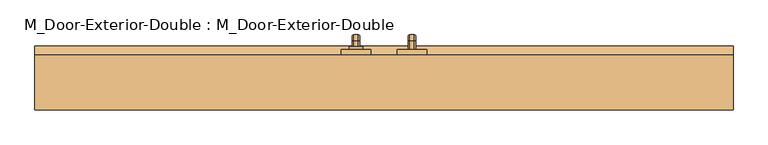
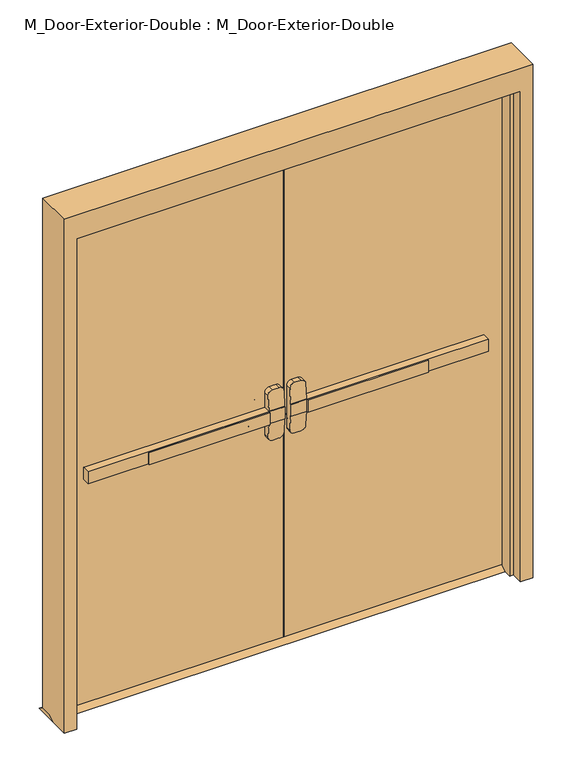
"""IFC4 building model written with IfcOpenShell, lengths in millimetres: door geometry, M_Door-Exterior-Double : M_Door-Exterior-Double."""

from ifc_helpers import new_model, si_unit, point, frame, frame_2d, origin, place, context, project, spatial, polyline, circle_curve, ellipse_curve, trimmed, segment, composite_curve, outline, extrude, faceted_brep, source, transform, mapped, element, save
from ifc_brep_helpers import plane_surface, cylinder_surface, revolved_surface, advanced_brep


def m_door_exterior_double_m_door_exterior_double_5cdccef0(model_context):
    return source(origin(), model_context, "Body", "SolidModel", [
        extrude(outline(polyline([(-566.1333333, -1.75), (-566.1333333, 4.6), (-76.2, 4.6), (-76.2, -1.75), (-566.1333333, -1.75)])), frame((0.0, 0.0, 974.6), z_axis=(0.0, 0.0, 1.0), x_axis=(1.0, 0.0, 0.0)), (0.0, 0.0, 1.0), 50.8),
        advanced_brep(
        [(-12.7, 4.6, 1025.4), (-76.2, 4.6, 1025.4), (-811.1, 4.6, 1025.4), (-811.1, 4.6, 974.6), (-76.2, 4.6, 974.6), (-12.7, 4.6, 974.6), (-811.1, 36.35, 1025.4), (-76.2, 36.35, 1025.4), (-76.2, 36.35, 1088.9), (-57.15, 36.35, 1107.95), (-31.75, 36.35, 1107.95), (-12.7, 36.35, 1088.9), (-12.7, 36.35, 911.1), (-31.75, 36.35, 892.05), (-57.15, 36.35, 892.05), (-76.2, 36.35, 911.1), (-76.2, 36.35, 974.6), (-811.1, 36.35, 974.6), (-12.7, 7.7752467, 1025.4), (-76.2, 7.7752467, 1025.4), (-12.7, 7.7752467, 974.6), (-12.7, 12.7854269, 911.1), (-12.7, 12.7854269, 1088.9), (-76.2, 7.7752467, 974.6), (-76.2, 12.7854269, 1088.9), (-76.2, 12.7854269, 911.1), (-57.15, 14.288481, 1107.95), (-31.75, 14.288481, 1107.95), (-31.75, 14.288481, 892.05), (-57.15, 14.288481, 892.05)],
        [
            (0, 1),
            (1, 2),
            (2, 3),
            (3, 4),
            (4, 5),
            (5, 0),
            (6, 7),
            (7, 8),
            (8, 9, circle_curve(frame((-57.15, 36.35, 1088.9), z_axis=(0.0, 1.0, 0.0), x_axis=(-1.0, 0.0, 0.0)), 19.05)),
            (9, 10),
            (10, 11, circle_curve(frame((-31.75, 36.35, 1088.9), z_axis=(0.0, 1.0, 0.0), x_axis=(-1.0, 0.0, 0.0)), 19.05)),
            (11, 12),
            (12, 13, circle_curve(frame((-31.75, 36.35, 911.1), z_axis=(0.0, 1.0, 0.0), x_axis=(-1.0, 0.0, 0.0)), 19.05)),
            (13, 14),
            (14, 15, circle_curve(frame((-57.15, 36.35, 911.1), z_axis=(0.0, 1.0, 0.0), x_axis=(-1.0, 0.0, 0.0)), 19.05)),
            (15, 16),
            (16, 17),
            (17, 6),
            (0, 18),
            (18, 19),
            (19, 7),
            (6, 2),
            (5, 20),
            (20, 21),
            (21, 12),
            (11, 22),
            (22, 18),
            (16, 23),
            (23, 20),
            (3, 17),
            (19, 24),
            (24, 8),
            (15, 25),
            (25, 23),
            (9, 26),
            (26, 27),
            (27, 10),
            (13, 28),
            (28, 29),
            (29, 14),
            (29, 25, ellipse_curve(frame((-57.15, 12.7854269, 911.1), z_axis=(0.0, 0.9969018152893365, 0.07865602756830282), x_axis=(0.0, -0.07865602756830208, 0.9969018152893365)), 19.1092038, 19.05)),
            (24, 26, ellipse_curve(frame((-57.15, 12.7854269, 1088.9), z_axis=(0.0, 0.9969018152893376, -0.07865602756828934), x_axis=(0.0, -0.078656027568288, -0.9969018152893377)), 19.1092038, 19.05)),
            (27, 22, ellipse_curve(frame((-31.75, 12.7854269, 1088.9), z_axis=(0.0, 0.9969018152893376, -0.07865602756828934), x_axis=(0.0, -0.078656027568288, -0.9969018152893377)), 19.1092038, 19.05)),
            (21, 28, ellipse_curve(frame((-31.75, 12.7854269, 911.1), z_axis=(0.0, 0.9969018152893365, 0.07865602756830282), x_axis=(0.0, -0.07865602756830208, 0.9969018152893365)), 19.1092038, 19.05)),
        ],
        [
            plane_surface(frame((-12.7, 4.6, 1025.4), z_axis=(0.0, -1.0, 0.0), x_axis=(1.0, 0.0, 0.0))),
            plane_surface(frame((-12.7, 36.35, 1025.4), z_axis=(0.0, 1.0, 0.0), x_axis=(-1.0, 0.0, 0.0))),
            plane_surface(frame((-811.1, 4.6, 1025.4), z_axis=(0.0, 0.0, 1.0), x_axis=(0.0, 1.0, 0.0))),
            plane_surface(frame((-12.7, 4.6, 1025.4), z_axis=(1.0, 0.0, 0.0), x_axis=(0.0, 1.0, 0.0))),
            plane_surface(frame((-12.7, 4.6, 974.6), z_axis=(0.0, 0.0, -1.0), x_axis=(0.0, 1.0, 0.0))),
            plane_surface(frame((-811.1, 4.6, 974.6), z_axis=(-1.0, 0.0, 0.0), x_axis=(0.0, 1.0, 0.0))),
            plane_surface(frame((-76.2, 7.7752467, 911.1), z_axis=(-1.0, 0.0, 0.0), x_axis=(0.0, 1.0, 0.0))),
            plane_surface(frame((-57.15, 7.7752467, 1107.95), z_axis=(0.0, 0.0, 1.0), x_axis=(0.0, 1.0, 0.0))),
            plane_surface(frame((-31.75, 7.7752467, 892.05), z_axis=(0.0, 0.0, -1.0), x_axis=(0.0, 1.0, 0.0))),
            cylinder_surface(frame((-57.15, 36.35, 911.1), z_axis=(0.0, -1.0, 0.0), x_axis=(-1.0, 0.0, 0.0)), 19.05),
            cylinder_surface(frame((-57.15, 36.35, 1088.9), z_axis=(0.0, -1.0, 0.0), x_axis=(-1.0, 0.0, 0.0)), 19.05),
            cylinder_surface(frame((-31.75, 36.35, 1088.9), z_axis=(0.0, -1.0, 0.0), x_axis=(-1.0, 0.0, 0.0)), 19.05),
            cylinder_surface(frame((-31.75, 36.35, 911.1), z_axis=(0.0, -1.0, 0.0), x_axis=(-1.0, 0.0, 0.0)), 19.05),
            plane_surface(frame((-76.2, 7.7752467, 1025.4), z_axis=(0.0, -0.9969018152893376, 0.07865602756828934), x_axis=(1.0, 0.0, 0.0))),
            plane_surface(frame((-76.2, 14.288481, 892.05), z_axis=(0.0, -0.9969018152893365, -0.07865602756830282), x_axis=(1.0, 0.0, 0.0))),
        ],
        [
            (0, [[1, 2, 3, 4, 5, 6]]),
            (1, [[7, 8, 9, 10, 11, 12, 13, 14, 15, 16, 17, 18]]),
            (2, [[-2, -1, 19, 20, 21, -7, 22]]),
            (3, [[23, 24, 25, -12, 26, 27, -19, -6]]),
            (4, [[-17, 28, 29, -23, -5, -4, 30]]),
            (5, [[-22, -18, -30, -3]]),
            (6, [[-21, 31, 32, -8]]),
            (6, [[33, 34, -28, -16]]),
            (7, [[35, 36, 37, -10]]),
            (8, [[38, 39, 40, -14]]),
            (9, [[-40, 41, -33, -15]]),
            (10, [[-32, 42, -35, -9]]),
            (11, [[-37, 43, -26, -11]]),
            (12, [[-25, 44, -38, -13]]),
            (13, [[-27, -43, -36, -42, -31, -20]]),
            (14, [[-29, -34, -41, -39, -44, -24]]),
        ],
    ),
        extrude(outline(polyline([(81.35, 15.0), (106.75, 0.0), (10.95, 0.0), (36.35, 15.0), (81.35, 15.0)])), frame((-950.0, 0.0, 0.0), z_axis=(1.0, 0.0, 0.0), x_axis=(0.0, 1.0, 0.0)), (0.0, 0.0, 1.0), 1900.0),
        extrude(outline(polyline([(566.1333333, -1.75), (76.2, -1.75), (76.2, 4.6), (566.1333333, 4.6), (566.1333333, -1.75)])), frame((0.0, 0.0, 974.6), z_axis=(0.0, 0.0, 1.0), x_axis=(1.0, 0.0, 0.0)), (0.0, 0.0, 1.0), 50.8),
        advanced_brep(
        [(12.7, 4.6, 1025.4), (12.7, 4.6, 974.6), (76.2, 4.6, 974.6), (811.1, 4.6, 974.6), (811.1, 4.6, 1025.4), (76.2, 4.6, 1025.4), (811.1, 36.35, 1025.4), (811.1, 36.35, 974.6), (76.2, 36.35, 974.6), (76.2, 36.35, 911.1), (57.15, 36.35, 892.05), (31.75, 36.35, 892.05), (12.7, 36.35, 911.1), (12.7, 36.35, 1088.9), (31.75, 36.35, 1107.95), (57.15, 36.35, 1107.95), (76.2, 36.35, 1088.9), (76.2, 36.35, 1025.4), (76.2, 7.7752467, 1025.4), (12.7, 7.7752467, 1025.4), (12.7, 12.7854269, 1088.9), (12.7, 12.7854269, 911.1), (12.7, 7.7752467, 974.6), (76.2, 7.7752467, 974.6), (76.2, 12.7854269, 911.1), (76.2, 12.7854269, 1088.9), (31.75, 14.288481, 1107.95), (57.15, 14.288481, 1107.95), (57.15, 14.288481, 892.05), (31.75, 14.288481, 892.05)],
        [
            (0, 1),
            (1, 2),
            (2, 3),
            (3, 4),
            (4, 5),
            (5, 0),
            (6, 7),
            (7, 8),
            (8, 9),
            (9, 10, circle_curve(frame((57.15, 36.35, 911.1), z_axis=(0.0, 1.0, 0.0), x_axis=(1.0, 0.0, 0.0)), 19.05)),
            (10, 11),
            (11, 12, circle_curve(frame((31.75, 36.35, 911.1), z_axis=(0.0, 1.0, 0.0), x_axis=(1.0, 0.0, 0.0)), 19.05)),
            (12, 13),
            (13, 14, circle_curve(frame((31.75, 36.35, 1088.9), z_axis=(0.0, 1.0, 0.0), x_axis=(1.0, 0.0, 0.0)), 19.05)),
            (14, 15),
            (15, 16, circle_curve(frame((57.15, 36.35, 1088.9), z_axis=(0.0, 1.0, 0.0), x_axis=(1.0, 0.0, 0.0)), 19.05)),
            (16, 17),
            (17, 6),
            (4, 6),
            (17, 18),
            (18, 19),
            (19, 0),
            (19, 20),
            (20, 13),
            (12, 21),
            (21, 22),
            (22, 1),
            (7, 3),
            (22, 23),
            (23, 8),
            (23, 24),
            (24, 9),
            (16, 25),
            (25, 18),
            (14, 26),
            (26, 27),
            (27, 15),
            (10, 28),
            (28, 29),
            (29, 11),
            (24, 28, ellipse_curve(frame((57.15, 12.7854269, 911.1), z_axis=(0.0, 0.9969018152893365, 0.07865602756830282), x_axis=(0.0, -0.07865602756830208, 0.9969018152893365)), 19.1092038, 19.05)),
            (27, 25, ellipse_curve(frame((57.15, 12.7854269, 1088.9), z_axis=(0.0, 0.9969018152893376, -0.07865602756828934), x_axis=(0.0, -0.078656027568288, -0.9969018152893377)), 19.1092038, 19.05)),
            (20, 26, ellipse_curve(frame((31.75, 12.7854269, 1088.9), z_axis=(0.0, 0.9969018152893376, -0.07865602756828934), x_axis=(0.0, -0.078656027568288, -0.9969018152893377)), 19.1092038, 19.05)),
            (29, 21, ellipse_curve(frame((31.75, 12.7854269, 911.1), z_axis=(0.0, 0.9969018152893365, 0.07865602756830282), x_axis=(0.0, -0.07865602756830208, 0.9969018152893365)), 19.1092038, 19.05)),
        ],
        [
            plane_surface(frame((12.7, 4.6, 1025.4), z_axis=(0.0, -1.0, 0.0), x_axis=(-1.0, 0.0, 0.0))),
            plane_surface(frame((12.7, 36.35, 1025.4), z_axis=(0.0, 1.0, 0.0), x_axis=(1.0, 0.0, 0.0))),
            plane_surface(frame((811.1, 4.6, 1025.4), z_axis=(0.0, 0.0, 1.0), x_axis=(0.0, 1.0, 0.0))),
            plane_surface(frame((12.7, 4.6, 1025.4), z_axis=(-1.0, 0.0, 0.0), x_axis=(0.0, 1.0, 0.0))),
            plane_surface(frame((12.7, 4.6, 974.6), z_axis=(0.0, 0.0, -1.0), x_axis=(0.0, 1.0, 0.0))),
            plane_surface(frame((811.1, 4.6, 974.6), z_axis=(1.0, 0.0, 0.0), x_axis=(0.0, 1.0, 0.0))),
            plane_surface(frame((76.2, 7.7752467, 911.1), z_axis=(1.0, 0.0, 0.0), x_axis=(0.0, 1.0, 0.0))),
            plane_surface(frame((57.15, 7.7752467, 1107.95), z_axis=(0.0, 0.0, 1.0), x_axis=(0.0, 1.0, 0.0))),
            plane_surface(frame((31.75, 7.7752467, 892.05), z_axis=(0.0, 0.0, -1.0), x_axis=(0.0, 1.0, 0.0))),
            cylinder_surface(frame((57.15, 36.35, 911.1), z_axis=(0.0, -1.0, 0.0), x_axis=(1.0, 0.0, 0.0)), 19.05),
            cylinder_surface(frame((57.15, 36.35, 1088.9), z_axis=(0.0, -1.0, 0.0), x_axis=(1.0, 0.0, 0.0)), 19.05),
            cylinder_surface(frame((31.75, 36.35, 1088.9), z_axis=(0.0, -1.0, 0.0), x_axis=(1.0, 0.0, 0.0)), 19.05),
            cylinder_surface(frame((31.75, 36.35, 911.1), z_axis=(0.0, -1.0, 0.0), x_axis=(1.0, 0.0, 0.0)), 19.05),
            plane_surface(frame((76.2, 7.7752467, 1025.4), z_axis=(0.0, -0.9969018152893376, 0.07865602756828934), x_axis=(-1.0, 0.0, 0.0))),
            plane_surface(frame((76.2, 14.288481, 892.05), z_axis=(0.0, -0.9969018152893365, -0.07865602756830282), x_axis=(-1.0, 0.0, 0.0))),
        ],
        [
            (0, [[1, 2, 3, 4, 5, 6]]),
            (1, [[7, 8, 9, 10, 11, 12, 13, 14, 15, 16, 17, 18]]),
            (2, [[19, -18, 20, 21, 22, -6, -5]]),
            (3, [[-1, -22, 23, 24, -13, 25, 26, 27]]),
            (4, [[28, -3, -2, -27, 29, 30, -8]]),
            (5, [[-4, -28, -7, -19]]),
            (6, [[-9, -30, 31, 32]]),
            (6, [[-17, 33, 34, -20]]),
            (7, [[-15, 35, 36, 37]]),
            (8, [[-11, 38, 39, 40]]),
            (9, [[-10, -32, 41, -38]]),
            (10, [[-16, -37, 42, -33]]),
            (11, [[-14, -24, 43, -35]]),
            (12, [[-12, -40, 44, -25]]),
            (13, [[-21, -34, -42, -36, -43, -23]]),
            (14, [[-26, -44, -39, -41, -31, -29]]),
        ],
    ),
        advanced_brep(
        [(66.2, 94.05, 1001.190625), (66.2, 94.05, 998.809375), (69.771875, 94.05, 995.2375), (82.6284594, 94.05, 995.2375), (86.2, 94.05, 998.8090406), (86.2, 94.05, 1001.190625), (82.628125, 94.05, 1004.7625), (69.771875, 94.05, 1004.7625), (66.2, 94.05, 874.609375), (69.771875, 94.05, 871.0375), (82.628125, 94.05, 871.0375), (86.2, 94.05, 874.609375), (86.2, 94.05, 876.9909594), (82.6284594, 94.05, 880.5625), (69.771875, 94.05, 880.5625), (66.2, 94.05, 876.990625), (66.2, 119.45, 1001.190625), (66.2, 133.340625, 987.3), (66.2, 133.340625, 888.5), (66.2, 119.45, 874.609375), (66.2, 119.45, 876.990625), (66.2, 130.959375, 888.5), (66.2, 130.959375, 987.3), (66.2, 119.45, 998.809375), (69.771875, 119.45, 995.2375), (82.6284594, 119.45, 995.2375), (86.2, 119.45, 998.8090406), (86.2, 130.9590406, 987.3), (86.2, 130.9590406, 888.5), (86.2, 119.45, 876.9909594), (86.2, 119.45, 874.609375), (86.2, 133.340625, 888.5), (86.2, 133.340625, 987.3), (86.2, 119.45, 1001.190625), (82.628125, 119.45, 1004.7625), (69.771875, 119.45, 1004.7625), (69.771875, 127.3875, 987.3), (82.6284594, 127.3875, 987.3), (82.628125, 136.9125, 987.3), (69.771875, 136.9125, 987.3), (69.771875, 127.3875, 888.5), (82.6284594, 127.3875, 888.5), (82.628125, 136.9125, 888.5), (69.771875, 136.9125, 888.5), (69.771875, 119.45, 880.5625), (82.6284594, 119.45, 880.5625), (82.628125, 119.45, 871.0375), (69.771875, 119.45, 871.0375)],
        [
            (0, 1),
            (1, 2, circle_curve(frame((69.771875, 94.05, 998.809375), z_axis=(0.0, -1.0, 0.0), x_axis=(0.0, 0.0, 1.0)), 3.571875)),
            (2, 3),
            (3, 4, circle_curve(frame((82.6284594, 94.05, 998.8090406), z_axis=(0.0, -1.0, 0.0), x_axis=(0.0, 0.0, 1.0)), 3.5715406)),
            (4, 5),
            (5, 6, circle_curve(frame((82.628125, 94.05, 1001.190625), z_axis=(0.0, -1.0, 0.0), x_axis=(0.0, 0.0, 1.0)), 3.571875)),
            (6, 7),
            (7, 0, circle_curve(frame((69.771875, 94.05, 1001.190625), z_axis=(0.0, -1.0, 0.0), x_axis=(0.0, 0.0, 1.0)), 3.571875)),
            (8, 9, circle_curve(frame((69.771875, 94.05, 874.609375), z_axis=(0.0, -1.0, 0.0), x_axis=(0.0, 0.0, -1.0)), 3.571875)),
            (9, 10),
            (10, 11, circle_curve(frame((82.628125, 94.05, 874.609375), z_axis=(0.0, -1.0, 0.0), x_axis=(0.0, 0.0, -1.0)), 3.571875)),
            (11, 12),
            (12, 13, circle_curve(frame((82.6284594, 94.05, 876.9909594), z_axis=(0.0, -1.0, 0.0), x_axis=(0.0, 0.0, -1.0)), 3.5715406)),
            (13, 14),
            (14, 15, circle_curve(frame((69.771875, 94.05, 876.990625), z_axis=(0.0, -1.0, 0.0), x_axis=(0.0, 0.0, -1.0)), 3.571875)),
            (15, 8),
            (0, 16),
            (16, 17, circle_curve(frame((66.2, 119.45, 987.3), z_axis=(-1.0, 0.0, 0.0), x_axis=(0.0, 0.0, 1.0)), 13.890625)),
            (17, 18),
            (18, 19, circle_curve(frame((66.2, 119.45, 888.5), z_axis=(-1.0, 0.0, 0.0), x_axis=(0.0, 1.0, 0.0)), 13.890625)),
            (19, 8),
            (15, 20),
            (20, 21, circle_curve(frame((66.2, 119.45, 888.5), z_axis=(1.0, 0.0, 0.0), x_axis=(0.0, 1.0, 0.0)), 11.509375)),
            (21, 22),
            (22, 23, circle_curve(frame((66.2, 119.45, 987.3), z_axis=(1.0, 0.0, 0.0), x_axis=(0.0, 0.0, 1.0)), 11.509375)),
            (23, 1),
            (23, 24, circle_curve(frame((69.771875, 119.45, 998.809375), z_axis=(0.0, -1.0, 0.0), x_axis=(0.0, 0.0, 1.0)), 3.571875)),
            (24, 2),
            (24, 25),
            (25, 3),
            (25, 26, circle_curve(frame((82.6284594, 119.45, 998.8090406), z_axis=(0.0, -1.0, 0.0), x_axis=(0.0, 0.0, 1.0)), 3.5715406)),
            (26, 4),
            (26, 27, circle_curve(frame((86.2, 119.45, 987.3), z_axis=(-1.0, 0.0, 0.0), x_axis=(0.0, 0.0, 1.0)), 11.5090406)),
            (27, 28),
            (28, 29, circle_curve(frame((86.2, 119.45, 888.5), z_axis=(-1.0, 0.0, 0.0), x_axis=(0.0, 1.0, 0.0)), 11.5090406)),
            (29, 12),
            (11, 30),
            (30, 31, circle_curve(frame((86.2, 119.45, 888.5), z_axis=(1.0, 0.0, 0.0), x_axis=(0.0, 1.0, 0.0)), 13.890625)),
            (31, 32),
            (32, 33, circle_curve(frame((86.2, 119.45, 987.3), z_axis=(1.0, 0.0, 0.0), x_axis=(0.0, 0.0, 1.0)), 13.890625)),
            (33, 5),
            (33, 34, circle_curve(frame((82.628125, 119.45, 1001.190625), z_axis=(0.0, -1.0, 0.0), x_axis=(0.0, 0.0, 1.0)), 3.571875)),
            (34, 6),
            (34, 35),
            (35, 7),
            (35, 16, circle_curve(frame((69.771875, 119.45, 1001.190625), z_axis=(0.0, -1.0, 0.0), x_axis=(0.0, 0.0, 1.0)), 3.571875)),
            (36, 24, circle_curve(frame((69.771875, 119.45, 987.3), z_axis=(1.0, 0.0, 0.0), x_axis=(0.0, 0.0, 1.0)), 7.9375)),
            (22, 36, circle_curve(frame((69.771875, 130.959375, 987.3), z_axis=(0.0, 0.0, 1.0), x_axis=(0.0, 1.0, 0.0)), 3.571875)),
            (37, 25, circle_curve(frame((82.6284594, 119.45, 987.3), z_axis=(1.0, 0.0, 0.0), x_axis=(0.0, 0.0, 1.0)), 7.9375)),
            (36, 37),
            (37, 27, circle_curve(frame((82.6284594, 130.9590406, 987.3), z_axis=(0.0, 0.0, 1.0), x_axis=(0.0, 1.0, 0.0)), 3.5715406)),
            (38, 34, circle_curve(frame((82.628125, 119.45, 987.3), z_axis=(1.0, 0.0, 0.0), x_axis=(0.0, 0.0, 1.0)), 17.4625)),
            (32, 38, circle_curve(frame((82.628125, 133.340625, 987.3), z_axis=(0.0, 0.0, 1.0), x_axis=(0.0, 1.0, 0.0)), 3.571875)),
            (39, 35, circle_curve(frame((69.771875, 119.45, 987.3), z_axis=(1.0, 0.0, 0.0), x_axis=(0.0, 0.0, 1.0)), 17.4625)),
            (38, 39),
            (39, 17, circle_curve(frame((69.771875, 133.340625, 987.3), z_axis=(0.0, 0.0, 1.0), x_axis=(0.0, 1.0, 0.0)), 3.571875)),
            (21, 40, circle_curve(frame((69.771875, 130.959375, 888.5), z_axis=(0.0, 0.0, 1.0), x_axis=(0.0, 1.0, 0.0)), 3.571875)),
            (40, 36),
            (40, 41),
            (41, 37),
            (41, 28, circle_curve(frame((82.6284594, 130.9590406, 888.5), z_axis=(0.0, 0.0, 1.0), x_axis=(0.0, 1.0, 0.0)), 3.5715406)),
            (31, 42, circle_curve(frame((82.628125, 133.340625, 888.5), z_axis=(0.0, 0.0, 1.0), x_axis=(0.0, 1.0, 0.0)), 3.571875)),
            (42, 38),
            (42, 43),
            (43, 39),
            (43, 18, circle_curve(frame((69.771875, 133.340625, 888.5), z_axis=(0.0, 0.0, 1.0), x_axis=(0.0, 1.0, 0.0)), 3.571875)),
            (44, 40, circle_curve(frame((69.771875, 119.45, 888.5), z_axis=(1.0, 0.0, 0.0), x_axis=(0.0, 1.0, 0.0)), 7.9375)),
            (20, 44, circle_curve(frame((69.771875, 119.45, 876.990625), z_axis=(0.0, 1.0, 0.0), x_axis=(0.0, 0.0, -1.0)), 3.571875)),
            (45, 41, circle_curve(frame((82.6284594, 119.45, 888.5), z_axis=(1.0, 0.0, 0.0), x_axis=(0.0, 1.0, 0.0)), 7.9375)),
            (44, 45),
            (45, 29, circle_curve(frame((82.6284594, 119.45, 876.9909594), z_axis=(0.0, 1.0, 0.0), x_axis=(0.0, 0.0, -1.0)), 3.5715406)),
            (46, 42, circle_curve(frame((82.628125, 119.45, 888.5), z_axis=(1.0, 0.0, 0.0), x_axis=(0.0, 1.0, 0.0)), 17.4625)),
            (30, 46, circle_curve(frame((82.628125, 119.45, 874.609375), z_axis=(0.0, 1.0, 0.0), x_axis=(0.0, 0.0, -1.0)), 3.571875)),
            (47, 43, circle_curve(frame((69.771875, 119.45, 888.5), z_axis=(1.0, 0.0, 0.0), x_axis=(0.0, 1.0, 0.0)), 17.4625)),
            (46, 47),
            (47, 19, circle_curve(frame((69.771875, 119.45, 874.609375), z_axis=(0.0, 1.0, 0.0), x_axis=(0.0, 0.0, -1.0)), 3.571875)),
            (14, 44),
            (13, 45),
            (10, 46),
            (9, 47),
        ],
        [
            plane_surface(frame((76.2, 94.05, 1000.0), z_axis=(0.0, -1.0, 0.0), x_axis=(1.0, 0.0, 0.0))),
            plane_surface(frame((76.2, 94.05, 875.8), z_axis=(0.0, -1.0, 0.0), x_axis=(1.0, 0.0, 0.0))),
            plane_surface(frame((66.2, 94.05, 1001.190625), z_axis=(-1.0, 0.0, 0.0), x_axis=(0.0, 1.0, 0.0))),
            cylinder_surface(frame((69.771875, 94.05, 998.809375), z_axis=(0.0, -1.0, 0.0), x_axis=(0.0, 0.0, 1.0)), 3.571875),
            plane_surface(frame((69.771875, 94.05, 995.2375), z_axis=(0.0, 0.0, -1.0), x_axis=(0.0, 1.0, 0.0))),
            cylinder_surface(frame((82.6284594, 94.05, 998.8090406), z_axis=(0.0, -1.0, 0.0), x_axis=(0.0, 0.0, 1.0)), 3.5715406),
            plane_surface(frame((86.2, 94.05, 998.8090406), z_axis=(1.0, 0.0, 0.0), x_axis=(0.0, 1.0, 0.0))),
            cylinder_surface(frame((82.628125, 94.05, 1001.190625), z_axis=(0.0, -1.0, 0.0), x_axis=(0.0, 0.0, 1.0)), 3.571875),
            plane_surface(frame((82.628125, 94.05, 1004.7625), z_axis=(0.0, 0.0, 1.0), x_axis=(0.0, 1.0, 0.0))),
            cylinder_surface(frame((69.771875, 94.05, 1001.190625), z_axis=(0.0, -1.0, 0.0), x_axis=(0.0, 0.0, 1.0)), 3.571875),
            revolved_surface(trimmed(ellipse_curve(frame((69.771875, 119.45, 998.809375), z_axis=(0.0, -1.0, 0.0), x_axis=(0.0, 0.0, 1.0)), 3.571875, 3.571875), [point((66.2, 119.45, 998.809375))], [point((69.771875, 119.45, 995.2375))], True, "CARTESIAN"), (76.2, 119.45, 987.3), (-1.0, 0.0, 0.0)),
            revolved_surface(polyline([(69.771875, 119.45, 995.2375), (82.6284594, 119.45, 995.2375)]), (76.2, 119.45, 987.3), (-1.0, 0.0, 0.0)),
            revolved_surface(trimmed(ellipse_curve(frame((82.6284594, 119.45, 998.8090406), z_axis=(0.0, -1.0, 0.0), x_axis=(0.0, 0.0, 1.0)), 3.5715406, 3.5715406), [point((82.6284594, 119.45, 995.2375))], [point((86.2, 119.45, 998.8090406))], True, "CARTESIAN"), (76.2, 119.45, 987.3), (-1.0, 0.0, 0.0)),
            revolved_surface(trimmed(ellipse_curve(frame((82.628125, 119.45, 1001.190625), z_axis=(0.0, -1.0, 0.0), x_axis=(0.0, 0.0, 1.0)), 3.571875, 3.571875), [point((86.2, 119.45, 1001.190625))], [point((82.628125, 119.45, 1004.7625))], True, "CARTESIAN"), (76.2, 119.45, 987.3), (-1.0, 0.0, 0.0)),
            cylinder_surface(frame((76.2, 119.45, 987.3), z_axis=(-1.0, 0.0, 0.0), x_axis=(0.0, 0.0, 1.0)), 17.4625),
            revolved_surface(trimmed(ellipse_curve(frame((69.771875, 119.45, 1001.190625), z_axis=(0.0, -1.0, 0.0), x_axis=(0.0, 0.0, 1.0)), 3.571875, 3.571875), [point((69.771875, 119.45, 1004.7625))], [point((66.2, 119.45, 1001.190625))], True, "CARTESIAN"), (76.2, 119.45, 987.3), (-1.0, 0.0, 0.0)),
            cylinder_surface(frame((69.771875, 130.959375, 987.3), z_axis=(0.0, 0.0, 1.0), x_axis=(0.0, 1.0, 0.0)), 3.571875),
            plane_surface(frame((69.771875, 127.3875, 987.3), z_axis=(0.0, -1.0, 0.0), x_axis=(0.0, 0.0, -1.0))),
            cylinder_surface(frame((82.6284594, 130.9590406, 987.3), z_axis=(0.0, 0.0, 1.0), x_axis=(0.0, 1.0, 0.0)), 3.5715406),
            cylinder_surface(frame((82.628125, 133.340625, 987.3), z_axis=(0.0, 0.0, 1.0), x_axis=(0.0, 1.0, 0.0)), 3.571875),
            plane_surface(frame((82.628125, 136.9125, 987.3), z_axis=(0.0, 1.0, 0.0), x_axis=(0.0, 0.0, -1.0))),
            cylinder_surface(frame((69.771875, 133.340625, 987.3), z_axis=(0.0, 0.0, 1.0), x_axis=(0.0, 1.0, 0.0)), 3.571875),
            revolved_surface(trimmed(ellipse_curve(frame((69.771875, 130.959375, 888.5), z_axis=(0.0, 0.0, 1.0), x_axis=(0.0, 1.0, 0.0)), 3.571875, 3.571875), [point((66.2, 130.959375, 888.5))], [point((69.771875, 127.3875, 888.5))], True, "CARTESIAN"), (76.2, 119.45, 888.5), (-1.0, 0.0, 0.0)),
            revolved_surface(polyline([(69.771875, 127.3875, 888.5), (82.6284594, 127.3875, 888.5)]), (76.2, 119.45, 888.5), (-1.0, 0.0, 0.0)),
            revolved_surface(trimmed(ellipse_curve(frame((82.6284594, 130.9590406, 888.5), z_axis=(0.0, 0.0, 1.0), x_axis=(0.0, 1.0, 0.0)), 3.5715406, 3.5715406), [point((82.6284594, 127.3875, 888.5))], [point((86.2, 130.9590406, 888.5))], True, "CARTESIAN"), (76.2, 119.45, 888.5), (-1.0, 0.0, 0.0)),
            revolved_surface(trimmed(ellipse_curve(frame((82.628125, 133.340625, 888.5), z_axis=(0.0, 0.0, 1.0), x_axis=(0.0, 1.0, 0.0)), 3.571875, 3.571875), [point((86.2, 133.340625, 888.5))], [point((82.628125, 136.9125, 888.5))], True, "CARTESIAN"), (76.2, 119.45, 888.5), (-1.0, 0.0, 0.0)),
            cylinder_surface(frame((76.2, 119.45, 888.5), z_axis=(-1.0, 0.0, 0.0), x_axis=(0.0, 1.0, 0.0)), 17.4625),
            revolved_surface(trimmed(ellipse_curve(frame((69.771875, 133.340625, 888.5), z_axis=(0.0, 0.0, 1.0), x_axis=(0.0, 1.0, 0.0)), 3.571875, 3.571875), [point((69.771875, 136.9125, 888.5))], [point((66.2, 133.340625, 888.5))], True, "CARTESIAN"), (76.2, 119.45, 888.5), (-1.0, 0.0, 0.0)),
            cylinder_surface(frame((69.771875, 119.45, 876.990625), z_axis=(0.0, 1.0, 0.0), x_axis=(0.0, 0.0, -1.0)), 3.571875),
            plane_surface(frame((69.771875, 119.45, 880.5625), z_axis=(0.0, 0.0, 1.0), x_axis=(0.0, -1.0, 0.0))),
            cylinder_surface(frame((82.6284594, 119.45, 876.9909594), z_axis=(0.0, 1.0, 0.0), x_axis=(0.0, 0.0, -1.0)), 3.5715406),
            cylinder_surface(frame((82.628125, 119.45, 874.609375), z_axis=(0.0, 1.0, 0.0), x_axis=(0.0, 0.0, -1.0)), 3.571875),
            plane_surface(frame((82.628125, 119.45, 871.0375), z_axis=(0.0, 0.0, -1.0), x_axis=(0.0, -1.0, 0.0))),
            cylinder_surface(frame((69.771875, 119.45, 874.609375), z_axis=(0.0, 1.0, 0.0), x_axis=(0.0, 0.0, -1.0)), 3.571875),
        ],
        [
            (0, [[1, 2, 3, 4, 5, 6, 7, 8]]),
            (1, [[9, 10, 11, 12, 13, 14, 15, 16]]),
            (2, [[-1, 17, 18, 19, 20, 21, -16, 22, 23, 24, 25, 26]]),
            (3, [[-2, -26, 27, 28]]),
            (4, [[-3, -28, 29, 30]]),
            (5, [[-4, -30, 31, 32]]),
            (6, [[-5, -32, 33, 34, 35, 36, -12, 37, 38, 39, 40, 41]]),
            (7, [[-6, -41, 42, 43]]),
            (8, [[-7, -43, 44, 45]]),
            (9, [[-8, -45, 46, -17]]),
            (10, [[47, -27, -25, 48]]),
            (11, [[49, -29, -47, 50]]),
            (12, [[-33, -31, -49, 51]]),
            (13, [[52, -42, -40, 53]]),
            (14, [[54, -44, -52, 55]]),
            (15, [[-18, -46, -54, 56]]),
            (16, [[-48, -24, 57, 58]]),
            (17, [[-50, -58, 59, 60]]),
            (18, [[-51, -60, 61, -34]]),
            (19, [[-53, -39, 62, 63]]),
            (20, [[-55, -63, 64, 65]]),
            (21, [[-56, -65, 66, -19]]),
            (22, [[67, -57, -23, 68]]),
            (23, [[69, -59, -67, 70]]),
            (24, [[-35, -61, -69, 71]]),
            (25, [[72, -62, -38, 73]]),
            (26, [[74, -64, -72, 75]]),
            (27, [[-20, -66, -74, 76]]),
            (28, [[-68, -22, -15, 77]]),
            (29, [[-70, -77, -14, 78]]),
            (30, [[-71, -78, -13, -36]]),
            (31, [[-73, -37, -11, 79]]),
            (32, [[-75, -79, -10, 80]]),
            (33, [[-76, -80, -9, -21]]),
        ],
    ),
        extrude(outline(composite_curve([segment(trimmed(circle_curve(frame_2d((1094.2338574, 76.2)), 90.1286291), [point((1175.0, 116.2))], [point((1175.0, 36.2))], False, "CARTESIAN"), True, "CONTINUOUS"), segment(polyline([(1175.0, 36.2), (825.0, 36.2)]), True, "CONTINUOUS"), segment(trimmed(circle_curve(frame_2d((905.7661426, 76.2)), 90.1286291), [point((825.0, 36.2))], [point((825.0, 116.2))], False, "CARTESIAN"), True, "CONTINUOUS"), segment(polyline([(825.0, 116.2), (1175.0, 116.2)]), True, "CONTINUOUS")], self_intersect=False)), frame((0.0, 81.35, 0.0), z_axis=(0.0, 1.0, 0.0), x_axis=(0.0, 0.0, 1.0)), (0.0, 0.0, 1.0), 15.0),
        advanced_brep(
        [(-86.2, 94.05, 1001.190625), (-86.2, 94.05, 998.809375), (-82.628125, 94.05, 995.2375), (-69.7715406, 94.05, 995.2375), (-66.2, 94.05, 998.8090406), (-66.2, 94.05, 1001.190625), (-69.771875, 94.05, 1004.7625), (-82.628125, 94.05, 1004.7625), (-86.2, 94.05, 874.609375), (-82.628125, 94.05, 871.0375), (-69.771875, 94.05, 871.0375), (-66.2, 94.05, 874.609375), (-66.2, 94.05, 876.9909594), (-69.7715406, 94.05, 880.5625), (-82.628125, 94.05, 880.5625), (-86.2, 94.05, 876.990625), (-86.2, 119.45, 1001.190625), (-86.2, 133.340625, 987.3), (-86.2, 133.340625, 888.5), (-86.2, 119.45, 874.609375), (-86.2, 119.45, 876.990625), (-86.2, 130.959375, 888.5), (-86.2, 130.959375, 987.3), (-86.2, 119.45, 998.809375), (-82.628125, 119.45, 995.2375), (-69.7715406, 119.45, 995.2375), (-66.2, 119.45, 998.8090406), (-66.2, 130.9590406, 987.3), (-66.2, 130.9590406, 888.5), (-66.2, 119.45, 876.9909594), (-66.2, 119.45, 874.609375), (-66.2, 133.340625, 888.5), (-66.2, 133.340625, 987.3), (-66.2, 119.45, 1001.190625), (-69.771875, 119.45, 1004.7625), (-82.628125, 119.45, 1004.7625), (-82.628125, 127.3875, 987.3), (-69.7715406, 127.3875, 987.3), (-69.771875, 136.9125, 987.3), (-82.628125, 136.9125, 987.3), (-82.628125, 127.3875, 888.5), (-69.7715406, 127.3875, 888.5), (-69.771875, 136.9125, 888.5), (-82.628125, 136.9125, 888.5), (-82.628125, 119.45, 880.5625), (-69.7715406, 119.45, 880.5625), (-69.771875, 119.45, 871.0375), (-82.628125, 119.45, 871.0375)],
        [
            (0, 1),
            (1, 2, circle_curve(frame((-82.628125, 94.05, 998.809375), z_axis=(0.0, -1.0, 0.0), x_axis=(0.0, 0.0, 1.0)), 3.571875)),
            (2, 3),
            (3, 4, circle_curve(frame((-69.7715406, 94.05, 998.8090406), z_axis=(0.0, -1.0, 0.0), x_axis=(0.0, 0.0, 1.0)), 3.5715406)),
            (4, 5),
            (5, 6, circle_curve(frame((-69.771875, 94.05, 1001.190625), z_axis=(0.0, -1.0, 0.0), x_axis=(0.0, 0.0, 1.0)), 3.571875)),
            (6, 7),
            (7, 0, circle_curve(frame((-82.628125, 94.05, 1001.190625), z_axis=(0.0, -1.0, 0.0), x_axis=(0.0, 0.0, 1.0)), 3.571875)),
            (8, 9, circle_curve(frame((-82.628125, 94.05, 874.609375), z_axis=(0.0, -1.0, 0.0), x_axis=(0.0, 0.0, -1.0)), 3.571875)),
            (9, 10),
            (10, 11, circle_curve(frame((-69.771875, 94.05, 874.609375), z_axis=(0.0, -1.0, 0.0), x_axis=(0.0, 0.0, -1.0)), 3.571875)),
            (11, 12),
            (12, 13, circle_curve(frame((-69.7715406, 94.05, 876.9909594), z_axis=(0.0, -1.0, 0.0), x_axis=(0.0, 0.0, -1.0)), 3.5715406)),
            (13, 14),
            (14, 15, circle_curve(frame((-82.628125, 94.05, 876.990625), z_axis=(0.0, -1.0, 0.0), x_axis=(0.0, 0.0, -1.0)), 3.571875)),
            (15, 8),
            (0, 16),
            (16, 17, circle_curve(frame((-86.2, 119.45, 987.3), z_axis=(-1.0, 0.0, 0.0), x_axis=(0.0, 0.0, 1.0)), 13.890625)),
            (17, 18),
            (18, 19, circle_curve(frame((-86.2, 119.45, 888.5), z_axis=(-1.0, 0.0, 0.0), x_axis=(0.0, 1.0, 0.0)), 13.890625)),
            (19, 8),
            (15, 20),
            (20, 21, circle_curve(frame((-86.2, 119.45, 888.5), z_axis=(1.0, 0.0, 0.0), x_axis=(0.0, 1.0, 0.0)), 11.509375)),
            (21, 22),
            (22, 23, circle_curve(frame((-86.2, 119.45, 987.3), z_axis=(1.0, 0.0, 0.0), x_axis=(0.0, 0.0, 1.0)), 11.509375)),
            (23, 1),
            (23, 24, circle_curve(frame((-82.628125, 119.45, 998.809375), z_axis=(0.0, -1.0, 0.0), x_axis=(0.0, 0.0, 1.0)), 3.571875)),
            (24, 2),
            (24, 25),
            (25, 3),
            (25, 26, circle_curve(frame((-69.7715406, 119.45, 998.8090406), z_axis=(0.0, -1.0, 0.0), x_axis=(0.0, 0.0, 1.0)), 3.5715406)),
            (26, 4),
            (26, 27, circle_curve(frame((-66.2, 119.45, 987.3), z_axis=(-1.0, 0.0, 0.0), x_axis=(0.0, 0.0, 1.0)), 11.5090406)),
            (27, 28),
            (28, 29, circle_curve(frame((-66.2, 119.45, 888.5), z_axis=(-1.0, 0.0, 0.0), x_axis=(0.0, 1.0, 0.0)), 11.5090406)),
            (29, 12),
            (11, 30),
            (30, 31, circle_curve(frame((-66.2, 119.45, 888.5), z_axis=(1.0, 0.0, 0.0), x_axis=(0.0, 1.0, 0.0)), 13.890625)),
            (31, 32),
            (32, 33, circle_curve(frame((-66.2, 119.45, 987.3), z_axis=(1.0, 0.0, 0.0), x_axis=(0.0, 0.0, 1.0)), 13.890625)),
            (33, 5),
            (33, 34, circle_curve(frame((-69.771875, 119.45, 1001.190625), z_axis=(0.0, -1.0, 0.0), x_axis=(0.0, 0.0, 1.0)), 3.571875)),
            (34, 6),
            (34, 35),
            (35, 7),
            (35, 16, circle_curve(frame((-82.628125, 119.45, 1001.190625), z_axis=(0.0, -1.0, 0.0), x_axis=(0.0, 0.0, 1.0)), 3.571875)),
            (36, 24, circle_curve(frame((-82.628125, 119.45, 987.3), z_axis=(1.0, 0.0, 0.0), x_axis=(0.0, 0.0, 1.0)), 7.9375)),
            (22, 36, circle_curve(frame((-82.628125, 130.959375, 987.3), z_axis=(0.0, 0.0, 1.0), x_axis=(0.0, 1.0, 0.0)), 3.571875)),
            (37, 25, circle_curve(frame((-69.7715406, 119.45, 987.3), z_axis=(1.0, 0.0, 0.0), x_axis=(0.0, 0.0, 1.0)), 7.9375)),
            (36, 37),
            (37, 27, circle_curve(frame((-69.7715406, 130.9590406, 987.3), z_axis=(0.0, 0.0, 1.0), x_axis=(0.0, 1.0, 0.0)), 3.5715406)),
            (38, 34, circle_curve(frame((-69.771875, 119.45, 987.3), z_axis=(1.0, 0.0, 0.0), x_axis=(0.0, 0.0, 1.0)), 17.4625)),
            (32, 38, circle_curve(frame((-69.771875, 133.340625, 987.3), z_axis=(0.0, 0.0, 1.0), x_axis=(0.0, 1.0, 0.0)), 3.571875)),
            (39, 35, circle_curve(frame((-82.628125, 119.45, 987.3), z_axis=(1.0, 0.0, 0.0), x_axis=(0.0, 0.0, 1.0)), 17.4625)),
            (38, 39),
            (39, 17, circle_curve(frame((-82.628125, 133.340625, 987.3), z_axis=(0.0, 0.0, 1.0), x_axis=(0.0, 1.0, 0.0)), 3.571875)),
            (21, 40, circle_curve(frame((-82.628125, 130.959375, 888.5), z_axis=(0.0, 0.0, 1.0), x_axis=(0.0, 1.0, 0.0)), 3.571875)),
            (40, 36),
            (40, 41),
            (41, 37),
            (41, 28, circle_curve(frame((-69.7715406, 130.9590406, 888.5), z_axis=(0.0, 0.0, 1.0), x_axis=(0.0, 1.0, 0.0)), 3.5715406)),
            (31, 42, circle_curve(frame((-69.771875, 133.340625, 888.5), z_axis=(0.0, 0.0, 1.0), x_axis=(0.0, 1.0, 0.0)), 3.571875)),
            (42, 38),
            (42, 43),
            (43, 39),
            (43, 18, circle_curve(frame((-82.628125, 133.340625, 888.5), z_axis=(0.0, 0.0, 1.0), x_axis=(0.0, 1.0, 0.0)), 3.571875)),
            (44, 40, circle_curve(frame((-82.628125, 119.45, 888.5), z_axis=(1.0, 0.0, 0.0), x_axis=(0.0, 1.0, 0.0)), 7.9375)),
            (20, 44, circle_curve(frame((-82.628125, 119.45, 876.990625), z_axis=(0.0, 1.0, 0.0), x_axis=(0.0, 0.0, -1.0)), 3.571875)),
            (45, 41, circle_curve(frame((-69.7715406, 119.45, 888.5), z_axis=(1.0, 0.0, 0.0), x_axis=(0.0, 1.0, 0.0)), 7.9375)),
            (44, 45),
            (45, 29, circle_curve(frame((-69.7715406, 119.45, 876.9909594), z_axis=(0.0, 1.0, 0.0), x_axis=(0.0, 0.0, -1.0)), 3.5715406)),
            (46, 42, circle_curve(frame((-69.771875, 119.45, 888.5), z_axis=(1.0, 0.0, 0.0), x_axis=(0.0, 1.0, 0.0)), 17.4625)),
            (30, 46, circle_curve(frame((-69.771875, 119.45, 874.609375), z_axis=(0.0, 1.0, 0.0), x_axis=(0.0, 0.0, -1.0)), 3.571875)),
            (47, 43, circle_curve(frame((-82.628125, 119.45, 888.5), z_axis=(1.0, 0.0, 0.0), x_axis=(0.0, 1.0, 0.0)), 17.4625)),
            (46, 47),
            (47, 19, circle_curve(frame((-82.628125, 119.45, 874.609375), z_axis=(0.0, 1.0, 0.0), x_axis=(0.0, 0.0, -1.0)), 3.571875)),
            (14, 44),
            (13, 45),
            (10, 46),
            (9, 47),
        ],
        [
            plane_surface(frame((-76.2, 94.05, 1000.0), z_axis=(0.0, -1.0, 0.0), x_axis=(1.0, 0.0, 0.0))),
            plane_surface(frame((-76.2, 94.05, 875.8), z_axis=(0.0, -1.0, 0.0), x_axis=(1.0, 0.0, 0.0))),
            plane_surface(frame((-86.2, 94.05, 1001.190625), z_axis=(-1.0, 0.0, 0.0), x_axis=(0.0, 1.0, 0.0))),
            cylinder_surface(frame((-82.628125, 94.05, 998.809375), z_axis=(0.0, -1.0, 0.0), x_axis=(0.0, 0.0, 1.0)), 3.571875),
            plane_surface(frame((-82.628125, 94.05, 995.2375), z_axis=(0.0, 0.0, -1.0), x_axis=(0.0, 1.0, 0.0))),
            cylinder_surface(frame((-69.7715406, 94.05, 998.8090406), z_axis=(0.0, -1.0, 0.0), x_axis=(0.0, 0.0, 1.0)), 3.5715406),
            plane_surface(frame((-66.2, 94.05, 998.8090406), z_axis=(1.0, 0.0, 0.0), x_axis=(0.0, 1.0, 0.0))),
            cylinder_surface(frame((-69.771875, 94.05, 1001.190625), z_axis=(0.0, -1.0, 0.0), x_axis=(0.0, 0.0, 1.0)), 3.571875),
            plane_surface(frame((-69.771875, 94.05, 1004.7625), z_axis=(0.0, 0.0, 1.0), x_axis=(0.0, 1.0, 0.0))),
            cylinder_surface(frame((-82.628125, 94.05, 1001.190625), z_axis=(0.0, -1.0, 0.0), x_axis=(0.0, 0.0, 1.0)), 3.571875),
            revolved_surface(trimmed(ellipse_curve(frame((-82.628125, 119.45, 998.809375), z_axis=(0.0, -1.0, 0.0), x_axis=(0.0, 0.0, 1.0)), 3.571875, 3.571875), [point((-86.2, 119.45, 998.809375))], [point((-82.628125, 119.45, 995.2375))], True, "CARTESIAN"), (-76.2, 119.45, 987.3), (-1.0, 0.0, 0.0)),
            revolved_surface(polyline([(-82.628125, 119.45, 995.2375), (-69.7715406, 119.45, 995.2375)]), (-76.2, 119.45, 987.3), (-1.0, 0.0, 0.0)),
            revolved_surface(trimmed(ellipse_curve(frame((-69.7715406, 119.45, 998.8090406), z_axis=(0.0, -1.0, 0.0), x_axis=(0.0, 0.0, 1.0)), 3.5715406, 3.5715406), [point((-69.7715406, 119.45, 995.2375))], [point((-66.2, 119.45, 998.8090406))], True, "CARTESIAN"), (-76.2, 119.45, 987.3), (-1.0, 0.0, 0.0)),
            revolved_surface(trimmed(ellipse_curve(frame((-69.771875, 119.45, 1001.190625), z_axis=(0.0, -1.0, 0.0), x_axis=(0.0, 0.0, 1.0)), 3.571875, 3.571875), [point((-66.2, 119.45, 1001.190625))], [point((-69.771875, 119.45, 1004.7625))], True, "CARTESIAN"), (-76.2, 119.45, 987.3), (-1.0, 0.0, 0.0)),
            cylinder_surface(frame((-76.2, 119.45, 987.3), z_axis=(-1.0, 0.0, 0.0), x_axis=(0.0, 0.0, 1.0)), 17.4625),
            revolved_surface(trimmed(ellipse_curve(frame((-82.628125, 119.45, 1001.190625), z_axis=(0.0, -1.0, 0.0), x_axis=(0.0, 0.0, 1.0)), 3.571875, 3.571875), [point((-82.628125, 119.45, 1004.7625))], [point((-86.2, 119.45, 1001.190625))], True, "CARTESIAN"), (-76.2, 119.45, 987.3), (-1.0, 0.0, 0.0)),
            cylinder_surface(frame((-82.628125, 130.959375, 987.3), z_axis=(0.0, 0.0, 1.0), x_axis=(0.0, 1.0, 0.0)), 3.571875),
            plane_surface(frame((-82.628125, 127.3875, 987.3), z_axis=(0.0, -1.0, 0.0), x_axis=(0.0, 0.0, -1.0))),
            cylinder_surface(frame((-69.7715406, 130.9590406, 987.3), z_axis=(0.0, 0.0, 1.0), x_axis=(0.0, 1.0, 0.0)), 3.5715406),
            cylinder_surface(frame((-69.771875, 133.340625, 987.3), z_axis=(0.0, 0.0, 1.0), x_axis=(0.0, 1.0, 0.0)), 3.571875),
            plane_surface(frame((-69.771875, 136.9125, 987.3), z_axis=(0.0, 1.0, 0.0), x_axis=(0.0, 0.0, -1.0))),
            cylinder_surface(frame((-82.628125, 133.340625, 987.3), z_axis=(0.0, 0.0, 1.0), x_axis=(0.0, 1.0, 0.0)), 3.571875),
            revolved_surface(trimmed(ellipse_curve(frame((-82.628125, 130.959375, 888.5), z_axis=(0.0, 0.0, 1.0), x_axis=(0.0, 1.0, 0.0)), 3.571875, 3.571875), [point((-86.2, 130.959375, 888.5))], [point((-82.628125, 127.3875, 888.5))], True, "CARTESIAN"), (-76.2, 119.45, 888.5), (-1.0, 0.0, 0.0)),
            revolved_surface(polyline([(-82.628125, 127.3875, 888.5), (-69.7715406, 127.3875, 888.5)]), (-76.2, 119.45, 888.5), (-1.0, 0.0, 0.0)),
            revolved_surface(trimmed(ellipse_curve(frame((-69.7715406, 130.9590406, 888.5), z_axis=(0.0, 0.0, 1.0), x_axis=(0.0, 1.0, 0.0)), 3.5715406, 3.5715406), [point((-69.7715406, 127.3875, 888.5))], [point((-66.2, 130.9590406, 888.5))], True, "CARTESIAN"), (-76.2, 119.45, 888.5), (-1.0, 0.0, 0.0)),
            revolved_surface(trimmed(ellipse_curve(frame((-69.771875, 133.340625, 888.5), z_axis=(0.0, 0.0, 1.0), x_axis=(0.0, 1.0, 0.0)), 3.571875, 3.571875), [point((-66.2, 133.340625, 888.5))], [point((-69.771875, 136.9125, 888.5))], True, "CARTESIAN"), (-76.2, 119.45, 888.5), (-1.0, 0.0, 0.0)),
            cylinder_surface(frame((-76.2, 119.45, 888.5), z_axis=(-1.0, 0.0, 0.0), x_axis=(0.0, 1.0, 0.0)), 17.4625),
            revolved_surface(trimmed(ellipse_curve(frame((-82.628125, 133.340625, 888.5), z_axis=(0.0, 0.0, 1.0), x_axis=(0.0, 1.0, 0.0)), 3.571875, 3.571875), [point((-82.628125, 136.9125, 888.5))], [point((-86.2, 133.340625, 888.5))], True, "CARTESIAN"), (-76.2, 119.45, 888.5), (-1.0, 0.0, 0.0)),
            cylinder_surface(frame((-82.628125, 119.45, 876.990625), z_axis=(0.0, 1.0, 0.0), x_axis=(0.0, 0.0, -1.0)), 3.571875),
            plane_surface(frame((-82.628125, 119.45, 880.5625), z_axis=(0.0, 0.0, 1.0), x_axis=(0.0, -1.0, 0.0))),
            cylinder_surface(frame((-69.7715406, 119.45, 876.9909594), z_axis=(0.0, 1.0, 0.0), x_axis=(0.0, 0.0, -1.0)), 3.5715406),
            cylinder_surface(frame((-69.771875, 119.45, 874.609375), z_axis=(0.0, 1.0, 0.0), x_axis=(0.0, 0.0, -1.0)), 3.571875),
            plane_surface(frame((-69.771875, 119.45, 871.0375), z_axis=(0.0, 0.0, -1.0), x_axis=(0.0, -1.0, 0.0))),
            cylinder_surface(frame((-82.628125, 119.45, 874.609375), z_axis=(0.0, 1.0, 0.0), x_axis=(0.0, 0.0, -1.0)), 3.571875),
        ],
        [
            (0, [[1, 2, 3, 4, 5, 6, 7, 8]]),
            (1, [[9, 10, 11, 12, 13, 14, 15, 16]]),
            (2, [[-1, 17, 18, 19, 20, 21, -16, 22, 23, 24, 25, 26]]),
            (3, [[-2, -26, 27, 28]]),
            (4, [[-3, -28, 29, 30]]),
            (5, [[-4, -30, 31, 32]]),
            (6, [[-5, -32, 33, 34, 35, 36, -12, 37, 38, 39, 40, 41]]),
            (7, [[-6, -41, 42, 43]]),
            (8, [[-7, -43, 44, 45]]),
            (9, [[-8, -45, 46, -17]]),
            (10, [[47, -27, -25, 48]]),
            (11, [[49, -29, -47, 50]]),
            (12, [[-33, -31, -49, 51]]),
            (13, [[52, -42, -40, 53]]),
            (14, [[54, -44, -52, 55]]),
            (15, [[-18, -46, -54, 56]]),
            (16, [[-48, -24, 57, 58]]),
            (17, [[-50, -58, 59, 60]]),
            (18, [[-51, -60, 61, -34]]),
            (19, [[-53, -39, 62, 63]]),
            (20, [[-55, -63, 64, 65]]),
            (21, [[-56, -65, 66, -19]]),
            (22, [[67, -57, -23, 68]]),
            (23, [[69, -59, -67, 70]]),
            (24, [[-35, -61, -69, 71]]),
            (25, [[72, -62, -38, 73]]),
            (26, [[74, -64, -72, 75]]),
            (27, [[-20, -66, -74, 76]]),
            (28, [[-68, -22, -15, 77]]),
            (29, [[-70, -77, -14, 78]]),
            (30, [[-71, -78, -13, -36]]),
            (31, [[-73, -37, -11, 79]]),
            (32, [[-75, -79, -10, 80]]),
            (33, [[-76, -80, -9, -21]]),
        ],
    ),
        extrude(outline(composite_curve([segment(trimmed(circle_curve(frame_2d((1098.8, -76.2)), 19.0), [point((1098.8, -95.2))], [point((1098.8, -57.2))], False, "CARTESIAN"), True, "CONTINUOUS"), segment(trimmed(circle_curve(frame_2d((1098.8, -76.2)), 19.0), [point((1098.8, -57.2))], [point((1098.8, -95.2))], False, "CARTESIAN"), True, "CONTINUOUS")], self_intersect=False)), frame((0.0, 96.35, 0.0), z_axis=(0.0, 1.0, 0.0), x_axis=(0.0, 0.0, 1.0)), (0.0, 0.0, 1.0), 8.73125),
        extrude(outline(composite_curve([segment(trimmed(circle_curve(frame_2d((1094.2338574, -76.2)), 90.1286291), [point((1175.0, -36.2))], [point((1175.0, -116.2))], False, "CARTESIAN"), True, "CONTINUOUS"), segment(polyline([(1175.0, -116.2), (825.0, -116.2)]), True, "CONTINUOUS"), segment(trimmed(circle_curve(frame_2d((905.7661426, -76.2)), 90.1286291), [point((825.0, -116.2))], [point((825.0, -36.2))], False, "CARTESIAN"), True, "CONTINUOUS"), segment(polyline([(825.0, -36.2), (1175.0, -36.2)]), True, "CONTINUOUS")], self_intersect=False)), frame((0.0, 81.35, 0.0), z_axis=(0.0, 1.0, 0.0), x_axis=(0.0, 0.0, 1.0)), (0.0, 0.0, 1.0), 15.0),
        faceted_brep([(900.0, 31.5875, 0.0), (900.0, 81.35, 0.0), (950.0, 81.35, 0.0), (950.0, -68.65, 0.0), (900.0, -68.65, 0.0), (900.0, -19.4375, 0.0), (884.125, -19.4375, 0.0), (884.125, 31.5875, 0.0), (900.0, 31.5875, 2100.0), (900.0, 81.35, 2100.0), (-900.0, 81.35, 2100.0), (-900.0, 81.35, 0.0), (-950.0, 81.35, 0.0), (-950.0, 81.35, 2200.0), (950.0, 81.35, 2200.0), (950.0, -68.65, 2200.0), (-950.0, -68.65, 2200.0), (-950.0, -68.65, 0.0), (-900.0, -68.65, 0.0), (-900.0, -68.65, 2100.0), (900.0, -68.65, 2100.0), (900.0, -19.4375, 2100.0), (-900.0, -19.4375, 2100.0), (-900.0, -19.4375, 0.0), (-884.125, -19.4375, 0.0), (-884.125, -19.4375, 2084.125), (884.125, -19.4375, 2084.125), (884.125, 31.5875, 2084.125), (-884.125, 31.5875, 2084.125), (-884.125, 31.5875, 0.0), (-900.0, 31.5875, 0.0), (-900.0, 31.5875, 2100.0)], [[[0, 1, 2, 3, 4, 5, 6, 7]], [[1, 0, 8, 9]], [[2, 1, 9, 10, 11, 12, 13, 14]], [[3, 2, 14, 15]], [[4, 3, 15, 16, 17, 18, 19, 20]], [[5, 4, 20, 21]], [[6, 5, 21, 22, 23, 24, 25, 26]], [[7, 6, 26, 27]], [[0, 7, 27, 28, 29, 30, 31, 8]], [[9, 8, 31, 10]], [[20, 19, 22, 21]], [[26, 25, 28, 27]], [[12, 11, 30, 29, 24, 23, 18, 17]], [[11, 10, 31, 30]], [[13, 12, 17, 16]], [[19, 18, 23, 22]], [[25, 24, 29, 28]], [[15, 14, 13, 16]]]),
        extrude(outline(polyline([(900.0, 36.35), (1.5875, 36.35), (1.5875, 81.35), (900.0, 81.35), (900.0, 36.35)])), frame((0.0, 0.0, 15.0), z_axis=(0.0, 0.0, 1.0), x_axis=(1.0, 0.0, 0.0)), (0.0, 0.0, 1.0), 2085.0),
        extrude(outline(polyline([(-1.5875, 36.35), (-900.0, 36.35), (-900.0, 81.35), (-1.5875, 81.35), (-1.5875, 36.35)])), frame((0.0, 0.0, 15.0), z_axis=(0.0, 0.0, 1.0), x_axis=(1.0, 0.0, 0.0)), (0.0, 0.0, 1.0), 2085.0),
    ])


if __name__ == "__main__":
    model = new_model("IFC4")
    model_context = context("Model", 3, world=origin())
    ifc_project = project(units=[si_unit("LENGTHUNIT", "METRE", prefix="MILLI")], contexts=[model_context])
    site = spatial("IfcSite", under=ifc_project)
    building = spatial("IfcBuilding", under=site)
    placement = place(None, origin())
    m_door_exterior_double_m_door_exterior_double_shape = m_door_exterior_double_m_door_exterior_double_5cdccef0(model_context)
    element("IfcDoor", 1, ObjectType="M_Door-Exterior-Double : M_Door-Exterior-Double", at=placement, inside=building, context=model_context, shape_type="MappedRepresentation", body=[
        mapped(m_door_exterior_double_m_door_exterior_double_shape, transform((0.0, 0.0, 0.0), x_axis=(1.0, 0.0, 0.0), y_axis=(0.0, 1.0, 0.0), z_axis=(0.0, 0.0, 1.0))),
    ])
    save(model, "model.ifc")

# Revit data of these elements
# Type "M_Door-Exterior-Double : M_Door-Exterior-Double"
#   Type Mark = "23"
#   Assembly Code = "B2030200"
#   Analytic Construction = "Metal"
#   Threshold Length [instance default] = 1900 mm
#   Threshold Offset [instance default] = 15 mm
#   Thickness = 45 mm
#   Thermal Resistance (R) = 0.270118 (m²·K)/W
#   Swing Angle [instance default] = 90.00°
#   Strike Height = 1000 mm
#   SinglePanelWidth = 900 mm
#   Rough Width [instance default] = 1900 mm
#   Rough Height [instance default] = 2200 mm
#   MFOpeningHeight [instance default] = 100 mm
#   MFOpeningWidth [instance default] = 100 mm
#   Inset Calculate [instance default] = 105 mm
#   Masonry Inset [instance default] = 25 mm
#   Height = 2100 mm
#   Width = 1800 mm
#   Heat Transfer Coefficient (U) = 3.70223 W/(m²·K)
#   Masonry Frame Depth = 150 mm
#   Threshold [instance default] = yes
#   Masonry Frame [instance default] = yes
#   Function = 1
#   Dry Wall Frame [instance default] = no
#   Threshold Material = Cherry
#   Panic Bar Material = Metal - Stainless Steel
#   Panel Material = Metal - Painted - Grey
#   Frame Material = Metal - Painted - Grey
#   Exterior Pull Material = Metal - Stainless Steel
#   Visual Light Transmittance = 0
#   Solar Heat Gain Coefficient = 0
#   Wall Closure = (empty or 0)
# Element 1 (IfcDoor, "M_Door-Exterior-Double : M_Door-Exterior-Double")
#   Materials on its faces: "Metal - Stainless Steel", "Metal - Painted - Grey", "Cherry"
# Materials
#   "Cherry": class "Wood", colour RGB 154 107 61, transparency 0, Description = "Prunus Serotina", Cost = 0
#   "Metal - Stainless Steel": class "Metal", colour RGB 247 247 247, transparency 0
#   "Metal - Painted - Grey": class "Paint", colour RGB 104 104 104, transparency 0, Cost = 0
